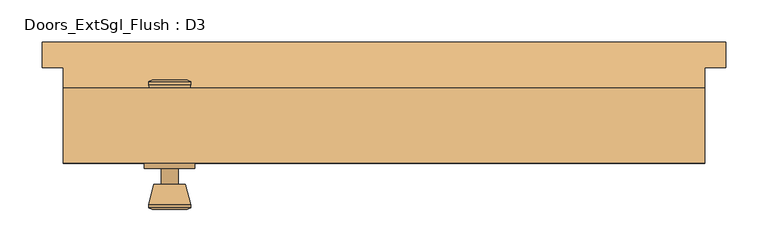
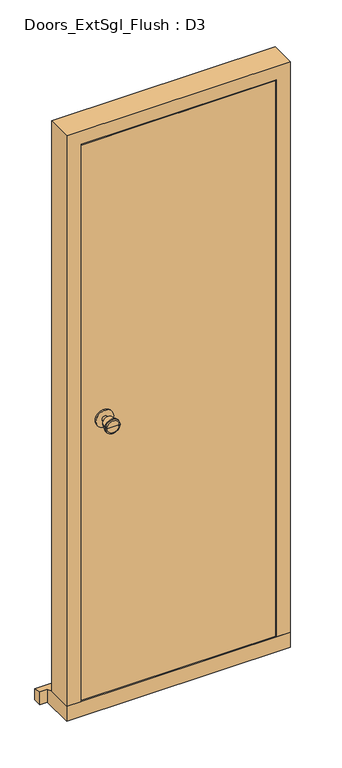
"""IFC4 building model written with IfcOpenShell, lengths in millimetres: door geometry, Doors_ExtSgl_Flush : D3."""

from ifc_helpers import new_model, si_unit, point, frame, frame_2d, origin, place, context, project, spatial, polyline, circle_curve, trimmed, segment, composite_curve, outline, extrude, faceted_brep, source, transform, mapped, element, save
from ifc_brep_helpers import plane_surface, cylinder_surface, revolved_surface, advanced_brep


def doors_extsgl_flush_d3_ba5ff989(model_context):
    return source(origin(), model_context, "Body", "SolidModel", [
        advanced_brep(
        [(-254.5, -43.8, 1050.0), (-244.5, -43.8, 1050.0), (-264.5, -43.8, 1050.0), (-234.0241324, -92.8, 1050.0), (-254.5, -92.8, 1050.0), (-274.9758676, -92.8, 1050.0), (-229.5, -90.9721319, 1050.0), (-279.5, -90.9721319, 1050.0), (-229.5, -87.5084537, 1050.0), (-279.5, -87.5084537, 1050.0), (-235.863764, -62.8, 1050.0), (-273.136236, -62.8, 1050.0), (-244.5, -62.8, 1050.0), (-264.5, -62.8, 1050.0)],
        [
            (0, 1),
            (1, 2, circle_curve(frame((-254.5, -43.8, 1050.0), z_axis=(0.0, 1.0, 0.0), x_axis=(-1.0, 0.0, 0.0)), 10.0)),
            (2, 0),
            (2, 1, circle_curve(frame((-254.5, -43.8, 1050.0), z_axis=(0.0, 1.0, 0.0), x_axis=(-1.0, 0.0, 0.0)), 10.0)),
            (3, 4),
            (4, 5),
            (5, 3, circle_curve(frame((-254.5, -92.8, 1050.0), z_axis=(0.0, -1.0, 0.0), x_axis=(-1.0, 0.0, 0.0)), 20.4758676)),
            (3, 5, circle_curve(frame((-254.5, -92.8, 1050.0), z_axis=(0.0, -1.0, 0.0), x_axis=(-1.0, 0.0, 0.0)), 20.4758676)),
            (6, 3),
            (5, 7),
            (7, 6, circle_curve(frame((-254.5, -90.9721319, 1050.0), z_axis=(0.0, -1.0, 0.0), x_axis=(-1.0, 0.0, 0.0)), 25.0)),
            (6, 7, circle_curve(frame((-254.5, -90.9721319, 1050.0), z_axis=(0.0, -1.0, 0.0), x_axis=(-1.0, 0.0, 0.0)), 25.0)),
            (8, 6),
            (7, 9),
            (9, 8, circle_curve(frame((-254.5, -87.5084537, 1050.0), z_axis=(0.0, -1.0, 0.0), x_axis=(-1.0, 0.0, 0.0)), 25.0)),
            (8, 9, circle_curve(frame((-254.5, -87.5084537, 1050.0), z_axis=(0.0, -1.0, 0.0), x_axis=(-1.0, 0.0, 0.0)), 25.0)),
            (10, 8),
            (9, 11),
            (11, 10, circle_curve(frame((-254.5, -62.8, 1050.0), z_axis=(0.0, -1.0, 0.0), x_axis=(-1.0, 0.0, 0.0)), 18.636236)),
            (10, 11, circle_curve(frame((-254.5, -62.8, 1050.0), z_axis=(0.0, -1.0, 0.0), x_axis=(-1.0, 0.0, 0.0)), 18.636236)),
            (12, 10),
            (11, 13),
            (13, 12, circle_curve(frame((-254.5, -62.8, 1050.0), z_axis=(0.0, -1.0, 0.0), x_axis=(-1.0, 0.0, 0.0)), 10.0)),
            (12, 13, circle_curve(frame((-254.5, -62.8, 1050.0), z_axis=(0.0, -1.0, 0.0), x_axis=(-1.0, 0.0, 0.0)), 10.0)),
            (1, 12),
            (13, 2),
        ],
        [
            plane_surface(frame((-254.5, -43.8, 1050.0), z_axis=(0.0, 1.0, 0.0), x_axis=(-1.0, 0.0, 0.0))),
            plane_surface(frame((-254.5, -92.8, 1050.0), z_axis=(0.0, -1.0, 0.0), x_axis=(-1.0, 0.0, 0.0))),
            revolved_surface(polyline([(-274.9758676, -92.8, 1050.0), (-279.5, -90.9721319, 1050.0)]), (-254.5, -43.8, 1050.0), (0.0, 1.0, 0.0)),
            cylinder_surface(frame((-254.5, -43.8, 1050.0), z_axis=(0.0, 1.0, 0.0), x_axis=(-1.0, 0.0, 0.0)), 25.0),
            revolved_surface(polyline([(-279.5, -87.5084537, 1050.0), (-273.136236, -62.8, 1050.0)]), (-254.5, -43.8, 1050.0), (0.0, 1.0, 0.0)),
            plane_surface(frame((-254.5, -62.8, 1050.0), z_axis=(0.0, 1.0, 0.0), x_axis=(-1.0, 0.0, 0.0))),
            cylinder_surface(frame((-254.5, -43.8, 1050.0), z_axis=(0.0, 1.0, 0.0), x_axis=(-1.0, 0.0, 0.0)), 10.0),
        ],
        [
            (0, [[1, 2, 3]]),
            (0, [[-3, 4, -1]]),
            (1, [[5, 6, 7]]),
            (1, [[-6, -5, 8]]),
            (2, [[9, -7, 10, 11]]),
            (2, [[-10, -8, -9, 12]]),
            (3, [[13, -11, 14, 15]]),
            (3, [[-14, -12, -13, 16]]),
            (4, [[17, -15, 18, 19]]),
            (4, [[-18, -16, -17, 20]]),
            (5, [[21, -19, 22, 23]]),
            (5, [[-22, -20, -21, 24]]),
            (6, [[25, -23, 26, -2]]),
            (6, [[-26, -24, -25, -4]]),
        ],
    ),
        extrude(outline(composite_curve([segment(trimmed(circle_curve(frame_2d((1050.0, -254.5)), 30.0), [point((1050.0, -284.5))], [point((1050.0, -224.5))], False, "CARTESIAN"), True, "CONTINUOUS"), segment(trimmed(circle_curve(frame_2d((1050.0, -254.5)), 30.0), [point((1050.0, -224.5))], [point((1050.0, -284.5))], False, "CARTESIAN"), True, "CONTINUOUS")], self_intersect=False)), frame((0.0, -43.8, 0.0), z_axis=(0.0, 1.0, 0.0), x_axis=(0.0, 0.0, 1.0)), (0.0, 0.0, 1.0), 6.0),
        advanced_brep(
        [(-254.5, 12.2, 1050.0), (-264.5, 12.2, 1050.0), (-244.5, 12.2, 1050.0), (-234.0241324, 61.2, 1050.0), (-274.9758676, 61.2, 1050.0), (-254.5, 61.2, 1050.0), (-229.5, 59.3721319, 1050.0), (-279.5, 59.3721319, 1050.0), (-229.5, 55.9084537, 1050.0), (-279.5, 55.9084537, 1050.0), (-235.863764, 31.2, 1050.0), (-273.136236, 31.2, 1050.0), (-244.5, 31.2, 1050.0), (-264.5, 31.2, 1050.0)],
        [
            (0, 1),
            (1, 2, circle_curve(frame((-254.5, 12.2, 1050.0), z_axis=(0.0, -1.0, 0.0), x_axis=(-1.0, 0.0, 0.0)), 10.0)),
            (2, 0),
            (2, 1, circle_curve(frame((-254.5, 12.2, 1050.0), z_axis=(0.0, -1.0, 0.0), x_axis=(-1.0, 0.0, 0.0)), 10.0)),
            (3, 4, circle_curve(frame((-254.5, 61.2, 1050.0), z_axis=(0.0, 1.0, 0.0), x_axis=(-1.0, 0.0, 0.0)), 20.4758676)),
            (4, 5),
            (5, 3),
            (4, 3, circle_curve(frame((-254.5, 61.2, 1050.0), z_axis=(0.0, 1.0, 0.0), x_axis=(-1.0, 0.0, 0.0)), 20.4758676)),
            (6, 7, circle_curve(frame((-254.5, 59.3721319, 1050.0), z_axis=(0.0, 1.0, 0.0), x_axis=(-1.0, 0.0, 0.0)), 25.0)),
            (7, 4),
            (3, 6),
            (7, 6, circle_curve(frame((-254.5, 59.3721319, 1050.0), z_axis=(0.0, 1.0, 0.0), x_axis=(-1.0, 0.0, 0.0)), 25.0)),
            (8, 9, circle_curve(frame((-254.5, 55.9084537, 1050.0), z_axis=(0.0, 1.0, 0.0), x_axis=(-1.0, 0.0, 0.0)), 25.0)),
            (9, 7),
            (6, 8),
            (9, 8, circle_curve(frame((-254.5, 55.9084537, 1050.0), z_axis=(0.0, 1.0, 0.0), x_axis=(-1.0, 0.0, 0.0)), 25.0)),
            (10, 11, circle_curve(frame((-254.5, 31.2, 1050.0), z_axis=(0.0, 1.0, 0.0), x_axis=(-1.0, 0.0, 0.0)), 18.636236)),
            (11, 9),
            (8, 10),
            (11, 10, circle_curve(frame((-254.5, 31.2, 1050.0), z_axis=(0.0, 1.0, 0.0), x_axis=(-1.0, 0.0, 0.0)), 18.636236)),
            (12, 13, circle_curve(frame((-254.5, 31.2, 1050.0), z_axis=(0.0, 1.0, 0.0), x_axis=(-1.0, 0.0, 0.0)), 10.0)),
            (13, 11),
            (10, 12),
            (13, 12, circle_curve(frame((-254.5, 31.2, 1050.0), z_axis=(0.0, 1.0, 0.0), x_axis=(-1.0, 0.0, 0.0)), 10.0)),
            (1, 13),
            (12, 2),
        ],
        [
            plane_surface(frame((-254.5, 12.2, 1050.0), z_axis=(0.0, -1.0, 0.0), x_axis=(-1.0, 0.0, 0.0))),
            plane_surface(frame((-254.5, 61.2, 1050.0), z_axis=(0.0, 1.0, 0.0), x_axis=(-1.0, 0.0, 0.0))),
            revolved_surface(polyline([(-274.9758676, 61.2, 1050.0), (-279.5, 59.3721319, 1050.0)]), (-254.5, 12.2, 1050.0), (0.0, -1.0, 0.0)),
            cylinder_surface(frame((-254.5, 12.2, 1050.0), z_axis=(0.0, -1.0, 0.0), x_axis=(-1.0, 0.0, 0.0)), 25.0),
            revolved_surface(polyline([(-279.5, 55.9084537, 1050.0), (-273.136236, 31.2, 1050.0)]), (-254.5, 12.2, 1050.0), (0.0, -1.0, 0.0)),
            plane_surface(frame((-254.5, 31.2, 1050.0), z_axis=(0.0, -1.0, 0.0), x_axis=(-1.0, 0.0, 0.0))),
            cylinder_surface(frame((-254.5, 12.2, 1050.0), z_axis=(0.0, -1.0, 0.0), x_axis=(-1.0, 0.0, 0.0)), 10.0),
        ],
        [
            (0, [[1, 2, 3]]),
            (0, [[-3, 4, -1]]),
            (1, [[5, 6, 7]]),
            (1, [[8, -7, -6]]),
            (2, [[9, 10, -5, 11]]),
            (2, [[12, -11, -8, -10]]),
            (3, [[13, 14, -9, 15]]),
            (3, [[16, -15, -12, -14]]),
            (4, [[17, 18, -13, 19]]),
            (4, [[20, -19, -16, -18]]),
            (5, [[21, 22, -17, 23]]),
            (5, [[24, -23, -20, -22]]),
            (6, [[-2, 25, -21, 26]]),
            (6, [[-4, -26, -24, -25]]),
        ],
    ),
        extrude(outline(composite_curve([segment(trimmed(circle_curve(frame_2d((1050.0, -254.5)), 30.0), [point((1050.0, -284.5))], [point((1050.0, -224.5))], False, "CARTESIAN"), True, "CONTINUOUS"), segment(trimmed(circle_curve(frame_2d((1050.0, -254.5)), 30.0), [point((1050.0, -224.5))], [point((1050.0, -284.5))], False, "CARTESIAN"), True, "CONTINUOUS")], self_intersect=False)), frame((0.0, 6.2, 0.0), z_axis=(0.0, 1.0, 0.0), x_axis=(0.0, 0.0, 1.0)), (0.0, 0.0, 1.0), 6.0),
        faceted_brep([(310.5, 51.2, 54.5), (381.0, 51.2, 54.5), (381.0, -37.8, 54.5), (332.5, -37.8, 54.5), (332.5, 9.2, 54.5), (310.5, 9.2, 54.5), (310.5, 51.2, 2039.5), (-310.5, 51.2, 2039.5), (-310.5, 51.2, 54.5), (-381.0, 51.2, 54.5), (-381.0, 51.2, 2110.0), (381.0, 51.2, 2110.0), (381.0, -37.8, 2110.0), (-381.0, -37.8, 2110.0), (-381.0, -37.8, 54.5), (-332.5, -37.8, 54.5), (-332.5, -37.8, 2061.5), (332.5, -37.8, 2061.5), (332.5, 9.2, 2061.5), (-332.5, 9.2, 2061.5), (-332.5, 9.2, 54.5), (-310.5, 9.2, 54.5), (-310.5, 9.2, 2039.5), (310.5, 9.2, 2039.5)], [[[0, 1, 2, 3, 4, 5]], [[1, 0, 6, 7, 8, 9, 10, 11]], [[2, 1, 11, 12]], [[3, 2, 12, 13, 14, 15, 16, 17]], [[4, 3, 17, 18]], [[5, 4, 18, 19, 20, 21, 22, 23]], [[0, 5, 23, 6]], [[7, 22, 21, 8]], [[8, 21, 20, 15, 14, 9]], [[13, 10, 9, 14]], [[19, 16, 15, 20]], [[12, 11, 10, 13]], [[18, 17, 16, 19]], [[6, 23, 22, 7]]]),
        extrude(outline(polyline([(329.5, -37.8), (-330.4250294, -37.8), (-330.4250294, 6.2), (329.5, 6.2), (329.5, -37.8)])), frame((0.0, 0.0, 58.5), z_axis=(0.0, 0.0, 1.0), x_axis=(1.0, 0.0, 0.0)), (0.0, 0.0, 1.0), 2000.0),
        faceted_brep([(406.0, 106.2, 0.0), (406.0, 106.2, 38.5947221), (406.0, 76.2, 47.2703282), (406.0, 76.2, 0.0), (-406.0, 106.2, 38.5947221), (-406.0, 106.2, 0.0), (-406.0, 76.2, 0.0), (-406.0, 76.2, 47.2703282), (381.0, 76.2, 0.0), (381.0, -37.8, 0.0), (-381.0, -37.8, 0.0), (-381.0, 76.2, 0.0), (-381.0, 76.2, 47.2703282), (-381.0, 51.2, 54.5), (381.0, 51.2, 54.5), (381.0, 76.2, 47.2703282), (-381.0, -37.8, 54.5), (381.0, -37.8, 54.5)], [[[0, 1, 2, 3]], [[4, 5, 6, 7]], [[5, 0, 3, 8, 9, 10, 11, 6]], [[1, 0, 5, 4]], [[1, 4, 7, 12, 13, 14, 15, 2]], [[13, 16, 17, 14]], [[16, 10, 9, 17]], [[12, 11, 10, 16, 13]], [[11, 12, 7, 6]], [[8, 15, 14, 17, 9]], [[15, 8, 3, 2]]]),
    ])


if __name__ == "__main__":
    model = new_model("IFC4")
    model_context = context("Model", 3, world=origin())
    ifc_project = project(units=[si_unit("LENGTHUNIT", "METRE", prefix="MILLI")], contexts=[model_context])
    site = spatial("IfcSite", under=ifc_project)
    building = spatial("IfcBuilding", under=site)
    placement = place(None, origin())
    doors_extsgl_flush_d3_shape = doors_extsgl_flush_d3_ba5ff989(model_context)
    element("IfcDoor", 1, ObjectType="Doors_ExtSgl_Flush : D3", at=placement, inside=building, context=model_context, shape_type="MappedRepresentation", body=[
        mapped(doors_extsgl_flush_d3_shape, transform((0.0, 0.0, 0.0), x_axis=(1.0, 0.0, 0.0), y_axis=(0.0, 1.0, 0.0), z_axis=(0.0, 0.0, 1.0))),
    ])
    save(model, "model.ifc")

# Revit data of these elements
# Type "Doors_ExtSgl_Flush : D3"
#   Type Mark = "51"
#   Type Comments = "External Single"
#   Operation = "SingleSwingRight"
#   Construction Type Id = "MDOOR"
#   Keynote = "L20"
#   Analytic Construction = "Metal"
#   Wrap Layers (Int) from Ext = 177.5 mm
#   Wrap Layers (Ext) from Ext = 102.5 mm
#   Thickness = 44 mm
#   Rough Width = 762 mm
#   Rough Height = 2110 mm
#   O/A Frame Width = 64 mm
#   Heat Transfer Coefficient (U) = 3.7021 W/(m²·K)
#   Handle Z Distance = 1050 mm
#   FrameWidth = 42 mm
#   FrameOffset - External = 25 mm
#   FrameDepth = 89 mm
#   Door Panel Width = 659 mm
#   Door Panel Thickness = 44 mm
#   Door Panel Height = 2000 mm
#   Cill Thickness = 54.5 mm
#   Cill Projection = 30 mm
#   Handle X Distance = 75 mm
#   Height = 2110 mm
#   Structural Tolerance = 6.5 mm
#   Tolerance = 3 mm
#   Undercut = 4 mm
#   Width = 762 mm
#   Cill Extension = 25 mm
#   Cavity Closer Width = 50 mm
#   Cavity Closer Offset from Ext = 102.5 mm
#   Cavity Closer Depth = 85 mm
#   Vis - Ironmongery = yes
#   Vis - Cavity Closers = yes
#   Define Thermal Properties by = 1
#   Function = 1
#   Material Door = Door - Panel
#   Material Frame = Door - Frame/Mullion
#   Material Ironmongery = Door - Handle
#   Visual Light Transmittance = 0
#   Solar Heat Gain Coefficient = 0
#   Wall Closure = (empty or 0)
# Element 1 (IfcDoor, "Doors_ExtSgl_Flush : D3")
#   Materials on its faces: "Door - Handle", "Door - Frame/Mullion", "Door - Panel"
# Materials
#   "Door - Panel": class "Wood", colour RGB 210 159 95, transparency 0, Keynote = "L20", Cost = 0
#   "Door - Frame/Mullion": class "Wood", colour RGB 212 179 113, transparency 0, Keynote = "L20", Cost = 0
#   "Door - Handle": colour RGB 0 0 0, transparency 0, Keynote = "P21", Cost = 0
